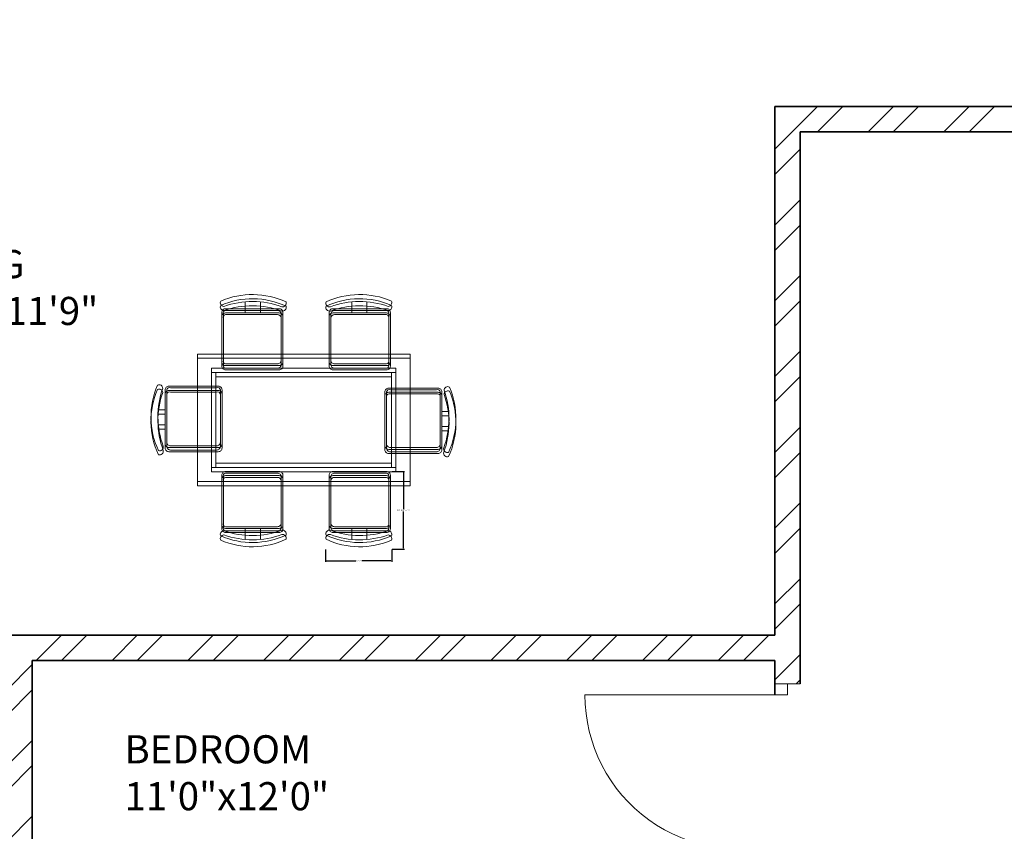
# Model space of a CAD drawing. Units: inches. Extents: x 1885 to 2748, y 783 to 2421.
# Tile 22 of 117: x 2163 to 2338, y 1206 to 1350. Entities that reach past the tile are written whole.
import ezdxf

# ---------------------------------------------------------------- set-up
doc = ezdxf.new("R2010")
doc.units = ezdxf.units.IN
for name, color, linetype, lineweight in [('A-ANNO-DIMS', 2, 'Continuous', 18), ('A-AREA-IDEN', 7, 'Continuous', 18), ('A-DOOR', 31, 'Continuous', 18), ('A-FURN', 8, 'Continuous', 13), ('A-WALL', 7, 'Continuous', 35)]:
    doc.layers.add(name, color=color, linetype=linetype, lineweight=lineweight)
doc.layers.add('A-WALL-PATT', color=85, linetype='Continuous', lineweight=13, true_color=0x58ba48)
doc.styles.get("Standard").update_dxf_attribs({"font": 'arial.ttf'})
doc.dimstyles.get("Standard").update_dxf_attribs({"dimtxt": 0.18, "dimasz": 0.18, "dimexe": 0.18, "dimexo": 0.0625, "dimgap": 0.09, "dimtad": 0, "dimtih": 1, "dimtoh": 1, "dimdec": 4, "dimzin": 0, "dimdsep": 46, "dimtxsty": 'Standard', "dimcen": 0.09, "dimadec": 0, "dimazin": 0, "dimtfac": 1, "dimtdec": 4, "dimtofl": 0, "dimtmove": 0, "dimatfit": 3, "dimfxl": 1, "dimtolj": 1, "dimtzin": 0, "dimarcsym": 0})

# ---------------------------------------------------------------- blocks, each defined once
blk = doc.blocks.new('TABLE-DINING-RECT')
for points in [[(0, 23.42), (37.78, 23.42), (37.78, 0.75), (0, 0.75)], [(0, 23.42), (37.78, 23.42), (37.78, 0.75), (0, 0.75)], [(0, 22.67), (37.78, 22.67), (37.78, 0), (0, 0)], [(0, 22.67), (37.78, 22.67), (37.78, 0), (0, 0)], [(2.51, 20.9), (35.26, 20.9), (35.26, 3.27), (2.51, 3.27)], [(2.51, 20.9), (35.26, 20.9), (35.26, 3.27), (2.51, 3.27)], [(2.51, 20.15), (35.26, 20.15), (35.26, 2.52), (2.51, 2.52)], [(2.51, 20.15), (35.26, 20.15), (35.26, 2.52), (2.51, 2.52)], [(3.27, 20.15), (34.5, 20.15), (34.5, 4.03), (3.27, 4.03)], [(3.27, 20.15), (34.5, 20.15), (34.5, 4.03), (3.27, 4.03)], [(3.27, 19.39), (34.5, 19.39), (34.5, 3.27), (3.27, 3.27)], [(3.27, 19.39), (34.5, 19.39), (34.5, 3.27), (3.27, 3.27)]]:
    blk.add_lwpolyline(points, close=True)
blk = doc.blocks.new('CHAIR-DINING-SIDE')
for points in [[(0.62, 11.29, -0.175809), (10.91, 11.21, 0.578392), (11.69, 12.07, 0.214524), (0.07, 12.23, 0.552014), (0.62, 11.29, -0.065079)], [(0.62, 11.29, -0.175809), (10.91, 11.21, 0.578392), (11.69, 12.07, 0.214524), (0.07, 12.23, 0.552014), (0.62, 11.29, -0.065079)], [(0.62, 10.54, -0.175809), (10.91, 10.46, 0.578392), (11.69, 11.32, 0.214524), (0.07, 11.47, 0.552014), (0.62, 10.54, -0.065079)], [(0.62, 10.54, -0.175809), (10.91, 10.46, 0.578392), (11.69, 11.32, 0.214524), (0.07, 11.47, 0.552014), (0.62, 10.54, -0.065079)], [(10.47, 10.88), (0.92, 10.88, 0.414214), (0.25, 10.21), (0.25, 1.43, 0.414214), (0.92, 0.76), (10.47, 0.76, 0.414214), (11.14, 1.43), (11.14, 10.21, 0.414214), (10.47, 10.88)], [(10.47, 10.88), (0.92, 10.88, 0.414214), (0.25, 10.21), (0.25, 1.43, 0.414214), (0.92, 0.76), (10.47, 0.76, 0.414214), (11.14, 1.43), (11.14, 10.21, 0.414214), (10.47, 10.88)], [(7.12, 10.88), (7.12, 12.09, -0.064759)], [(7.12, 10.88), (7.12, 12.09, -0.064759)], [(7.12, 10.12), (7.12, 11.33, -0.064759)], [(7.12, 10.12), (7.12, 11.33, -0.064759)], [(10.47, 10.12), (0.92, 10.12, 0.414214), (0.25, 9.46), (0.25, 0.67, 0.414214), (0.92, 0), (10.47, 0, 0.414214), (11.14, 0.67), (11.14, 9.46, 0.414214), (10.47, 10.12)], [(10.47, 10.12), (0.92, 10.12, 0.414214), (0.25, 9.46), (0.25, 0.67, 0.414214), (0.92, 0), (10.47, 0, 0.414214), (11.14, 0.67), (11.14, 9.46, 0.414214), (10.47, 10.12)]]:
    blk.add_lwpolyline(points, format="xyb")
for points in [[(0.92, 10.58), (10.17, 10.58, -0.414214), (10.84, 9.91), (10.84, 1.73, -0.414214), (10.17, 1.06), (0.92, 1.06, -0.512069), (0.55, 1.73), (0.55, 9.91, -0.512069)], [(0.92, 10.58), (10.17, 10.58, -0.414214), (10.84, 9.91), (10.84, 1.73, -0.414214), (10.17, 1.06), (0.92, 1.06, -0.512069), (0.55, 1.73), (0.55, 9.91, -0.512069)], [(0.92, 9.82), (10.17, 9.82, -0.414214), (10.84, 9.15), (10.84, 0.97, -0.414214), (10.17, 0.3), (0.92, 0.3, -0.512069), (0.55, 0.97), (0.55, 9.15, -0.512069)], [(0.92, 9.82), (10.17, 9.82, -0.414214), (10.84, 9.15), (10.84, 0.97, -0.414214), (10.17, 0.3), (0.92, 0.3, -0.512069), (0.55, 0.97), (0.55, 9.15, -0.512069)]]:
    blk.add_lwpolyline(points, format="xyb", close=True)
for points in [[(4.44, 12.11), (4.44, 10.88)], [(4.44, 12.11), (4.44, 10.88)], [(4.44, 11.35), (4.44, 10.12)], [(4.44, 11.35), (4.44, 10.12)]]:
    blk.add_lwpolyline(points)
blk = doc.blocks.new('CHAIR-DINING-SIDE-B')
for points in [[(10.8, 3.27, 0.414214), (11.47, 3.94), (11.47, 12.73, 0.414214), (10.8, 13.39), (1.25, 13.39, 0.414214), (0.58, 12.73), (0.58, 3.94, 0.414214), (1.25, 3.27), (10.8, 3.27)], [(10.8, 3.27, 0.414214), (11.47, 3.94), (11.47, 12.73, 0.414214), (10.8, 13.39), (1.25, 13.39, 0.414214), (0.58, 12.73), (0.58, 3.94, 0.414214), (1.25, 3.27), (10.8, 3.27)], [(10.8, 2.52, 0.414214), (11.47, 3.19), (11.47, 11.97, 0.414214), (10.8, 12.64), (1.25, 12.64, 0.414214), (0.58, 11.97), (0.58, 3.19, 0.414214), (1.25, 2.52), (10.8, 2.52)], [(10.8, 2.52, 0.414214), (11.47, 3.19), (11.47, 11.97, 0.414214), (10.8, 12.64), (1.25, 12.64, 0.414214), (0.58, 11.97), (0.58, 3.19, 0.414214), (1.25, 2.52), (10.8, 2.52)], [(11.1, 2.86, -0.175809), (0.81, 2.94, 0.578392), (0.03, 2.08, 0.214524), (11.65, 1.93, 0.552014), (11.1, 2.86, -0.065079)], [(11.1, 2.86, -0.175809), (0.81, 2.94, 0.578392), (0.03, 2.08, 0.214524), (11.65, 1.93, 0.552014), (11.1, 2.86, -0.065079)], [(11.1, 2.11, -0.175809), (0.81, 2.18, 0.578392), (0.03, 1.33, 0.214524), (11.65, 1.17, 0.552014), (11.1, 2.11, -0.065079)], [(11.1, 2.1, -0.175809), (0.81, 2.18, 0.578392), (0.03, 1.33, 0.214524), (11.65, 1.17, 0.552014), (11.1, 2.1, -0.065079)], [(4.6, 3.27), (4.6, 2.07, -0.064759)], [(4.6, 3.27), (4.6, 2.07, -0.064759)], [(4.6, 2.52), (4.6, 1.31, -0.064759)], [(4.6, 2.52), (4.6, 1.31, -0.064759)]]:
    blk.add_lwpolyline(points, format="xyb")
for points in [[(10.8, 3.57), (1.55, 3.57, -0.414214), (0.88, 4.24), (0.88, 12.42, -0.414214), (1.55, 13.09), (10.8, 13.09, -0.512069), (11.17, 12.42), (11.17, 4.24, -0.512069)], [(10.8, 3.57), (1.55, 3.57, -0.414214), (0.88, 4.24), (0.88, 12.42, -0.414214), (1.55, 13.09), (10.8, 13.09, -0.512069), (11.17, 12.42), (11.17, 4.24, -0.512069)], [(10.8, 2.82), (1.55, 2.82, -0.414214), (0.88, 3.49), (0.88, 11.67, -0.414214), (1.55, 12.34), (10.8, 12.34, -0.512069), (11.17, 11.67), (11.17, 3.49, -0.512069)], [(10.8, 2.82), (1.55, 2.82, -0.414214), (0.88, 3.49), (0.88, 11.67, -0.414214), (1.55, 12.34), (10.8, 12.34, -0.512069), (11.17, 11.67), (11.17, 3.49, -0.512069)]]:
    blk.add_lwpolyline(points, format="xyb", close=True)
for points in [[(7.28, 2.04), (7.28, 3.27)], [(7.28, 2.04), (7.28, 3.27)], [(7.28, 1.29), (7.28, 2.52)], [(7.28, 1.29), (7.28, 2.52)]]:
    blk.add_lwpolyline(points)
blk = doc.blocks.new('*D39')
at = {"layer": 'A-ANNO-DIMS', "color": 0, "lineweight": -2, "transparency": 16777216}
for p, q in [((2228.76, 1269.64), (2230.95, 1269.64)), ((2230.77, 1269.46), (2230.77, 1262.91)), ((2230.77, 1255.99), (2230.77, 1262.54)), ((2228.76, 1255.81), (2230.95, 1255.81))]:
    blk.add_line(p, q, dxfattribs=at)
at = {"layer": 'A-ANNO-DIMS', "color": 0, "transparency": 16777216}
for points in [[(2230.74, 1269.46), (2230.8, 1269.46), (2230.77, 1269.64)], [(2230.74, 1255.99), (2230.8, 1255.99), (2230.77, 1255.81)]]:
    blk.add_solid(points, dxfattribs=at)
at = {"layer": 'Defpoints', "color": 0, "transparency": 16777216}
for p in [(2228.7, 1269.64), (2230.77, 1269.64), (2228.7, 1255.81)]:
    blk.add_point(p, dxfattribs=at)
at = {"layer": 'A-ANNO-DIMS', "color": 0, "transparency": 16777216, "insert": (2230.77, 1262.73), "char_height": 0.18, "attachment_point": 5}
blk.add_mtext('\\A1;SIDE CHAIR B 14 TYP.', dxfattribs=at)
blk = doc.blocks.new('*D40')
at = {"layer": 'A-ANNO-DIMS', "color": 0, "lineweight": -2, "transparency": 16777216}
for p, q in [((2216.91, 1255.75), (2216.91, 1253.55)), ((2228.7, 1255.75), (2228.7, 1253.55)), ((2217.09, 1253.73), (2222.28, 1253.73)), ((2228.52, 1253.73), (2223.32, 1253.73))]:
    blk.add_line(p, q, dxfattribs=at)
at = {"layer": 'A-ANNO-DIMS', "color": 0, "transparency": 16777216}
for points in [[(2217.09, 1253.76), (2217.09, 1253.7), (2216.91, 1253.73)], [(2228.52, 1253.76), (2228.52, 1253.7), (2228.7, 1253.73)]]:
    blk.add_solid(points, dxfattribs=at)
at = {"layer": 'Defpoints', "color": 0, "transparency": 16777216}
for p in [(2216.91, 1255.81), (2228.7, 1255.81), (2228.7, 1253.73)]:
    blk.add_point(p, dxfattribs=at)
at = {"layer": 'A-ANNO-DIMS', "color": 0, "transparency": 16777216, "insert": (2222.8, 1253.73), "char_height": 0.18, "attachment_point": 5}
blk.add_mtext('\\A1;12 TYP.', dxfattribs=at)

msp = doc.modelspace()

# ---------------------------------------------------------------- hatches: boundary and pattern name
at = {"layer": 'A-WALL-PATT'}
h = msp.add_hatch(dxfattribs=at)
h.set_pattern_fill('ANSI32', color=256)
h.paths.add_polyline_path([(2007.77, 2318.01), (1980.77, 2318.01), (1980.77, 2281.22), (1985.27, 2281.22), (1985.27, 2313.51), (2007.77, 2313.51), (2007.77, 2315.76)])
h.paths.add_polyline_path([(2094.32, 2318.01), (2067.77, 2318.01), (2067.77, 2313.51), (2094.32, 2313.51), (2094.32, 2315.76)])
h.paths.add_polyline_path([(2131.37, 2315.76), (2131.37, 2318.01), (2131.19, 2318.01), (2112.61, 2318.01), (2112.61, 2313.51), (2117.27, 2313.51), (2117.27, 2255.2), (2121.77, 2255.2), (2121.77, 2313.51), (2131.37, 2313.51)])
h.paths.add_polyline_path([(2190.51, 2318.01), (2155.37, 2318.01), (2155.37, 2313.51), (2169.77, 2313.51), (2169.77, 2229.51), (2121.77, 2229.51), (2121.77, 2233.45), (2119.52, 2233.45), (2117.27, 2233.45), (2117.27, 2201.1), (2121.77, 2201.1), (2121.77, 2225.01), (2169.77, 2225.01), (2169.77, 2165.01), (2306.27, 2165.01), (2306.27, 2066.01), (2310.77, 2066.01), (2344.27, 2066.01), (2486.27, 2066.01), (2486.27, 1886.01), (2483.02, 1886.01), (2483.02, 1881.51), (2486.27, 1881.51), (2486.27, 1880.68), (2490.77, 1880.68), (2490.77, 2070.51), (2344.27, 2070.51), (2310.77, 2070.51), (2310.77, 2165.01), (2310.77, 2173.64), (2308.52, 2173.64), (2306.27, 2173.64), (2306.27, 2169.51), (2174.27, 2169.51), (2174.27, 2313.51), (2190.51, 2313.51), (2190.51, 2315.76)])
h.paths.add_polyline_path([(1985.27, 2221.22), (1980.77, 2221.22), (1980.77, 2165.01), (1992.77, 2165.01), (1992.77, 2141.93), (1997.27, 2141.93), (1997.27, 2165.01), (2117.27, 2165.01), (2117.27, 2163.13), (2121.77, 2163.13), (2121.77, 2172.73), (2119.52, 2172.73), (2117.27, 2172.73), (2117.27, 2169.51), (1985.27, 2169.51)])
h.paths.add_polyline_path([(1997.27, 2105.93), (1992.77, 2105.93), (1992.77, 2070.51), (2016.77, 2070.51), (2016.77, 2059.12), (2019.02, 2059.12), (2021.27, 2059.12), (2021.27, 2070.51), (2117.27, 2070.51), (2117.27, 2022.51), (2114.42, 2022.51), (2114.42, 2018.01), (2123.63, 2018.01), (2123.63, 2020.26), (2123.63, 2022.51), (2121.77, 2022.51), (2121.77, 2142.59), (2119.52, 2142.59), (2117.27, 2142.59), (2117.27, 2075.01), (1997.27, 2075.01)])
h.paths.add_polyline_path([(2092.03, 2020.26), (2092.03, 2022.51), (2021.27, 2022.51), (2021.27, 2035.12), (2016.77, 2035.12), (2016.77, 2018.01), (2016.77, 1978.78), (2021.27, 1978.78), (2021.27, 2018.01), (2092.03, 2018.01)])
h.paths.add_polyline_path([(2260.94, 2022.51), (2153.1, 2022.51), (2153.1, 2020.26), (2153.1, 2018.01), (2155.27, 2018.01), (2155.27, 1886.01), (2107.63, 1886.01), (2107.63, 1881.51), (2182.91, 1881.51), (2182.91, 1883.76), (2182.91, 1886.01), (2159.77, 1886.01), (2159.77, 2018.01), (2260.94, 2018.01), (2260.94, 2020.26)])
h.paths.add_polyline_path([(2047.63, 1883.76), (2047.63, 1886.01), (2021.27, 1886.01), (2021.27, 1918.78), (2019.02, 1918.78), (2016.77, 1918.78), (2016.77, 1881.51), (2047.63, 1881.51)])
h.paths.add_polyline_path([(2306.36, 1883.76), (2306.36, 1886.01), (2296.27, 1886.01), (2296.27, 1982.01), (2316.54, 1982.01), (2316.54, 1984.26), (2316.54, 1986.51), (2296.27, 1986.51), (2296.27, 2022.51), (2289.28, 2022.51), (2289.28, 2018.01), (2291.77, 2018.01), (2291.77, 1886.01), (2242.91, 1886.01), (2242.91, 1881.51), (2306.36, 1881.51)], flags=17)
h.paths.add_polyline_path([(1985.27, 1843.01), (2021.6, 1843.01), (2021.53, 1845.44), (2021.48, 1847.51), (1980.77, 1847.51), (1980.77, 1809.45), (1985.27, 1809.45)])
h.paths.add_polyline_path([(2131.48, 1845.26), (2131.48, 1847.51), (2081.53, 1847.51), (2081.53, 1843.01), (2117.27, 1843.01), (2117.27, 1784.15), (2119.52, 1784.15), (2121.77, 1784.15), (2121.77, 1843.01), (2131.48, 1843.01)])
h.paths.add_polyline_path([(2203.89, 1847.51), (2155.48, 1847.51), (2155.48, 1843.01), (2169.77, 1843.01), (2169.77, 1759.01), (2121.77, 1759.01), (2121.77, 1761.46), (2117.27, 1761.46), (2117.27, 1730.43), (2121.77, 1730.43), (2121.77, 1754.51), (2177.42, 1754.51), (2177.42, 1756.76), (2177.42, 1759.01), (2174.27, 1759.01), (2174.27, 1843.01), (2203.89, 1843.01)])
h.paths.add_polyline_path([(2335.55, 1845.26), (2335.55, 1847.51), (2239.89, 1847.51), (2239.89, 1843.01), (2306.27, 1843.01), (2306.27, 1759.01), (2199.49, 1759.01), (2199.49, 1754.51), (2310.77, 1754.51), (2310.77, 1843.01), (2335.55, 1843.01)])
h.paths.add_polyline_path([(2348.77, 2022.51), (2344.27, 2022.51), (2344.27, 1986.51), (2341.68, 1986.51), (2341.68, 1982.01), (2344.27, 1982.01), (2344.27, 1886.01), (2330.36, 1886.01), (2330.36, 1881.51), (2361.63, 1881.51), (2361.63, 1883.76), (2361.63, 1886.01), (2348.77, 1886.01)], flags=17)
h.paths.add_polyline_path([(2283.25, 2315.76), (2283.25, 2318.01), (2238.51, 2318.01), (2238.51, 2313.51), (2283.25, 2313.51)], flags=17)
h.paths.add_polyline_path([(2363.27, 2348.01), (2388.68, 2348.01), (2388.68, 2350.26), (2388.68, 2352.51), (2358.77, 2352.51), (2358.77, 2348.01), (2358.77, 2318.01), (2344.48, 2318.01), (2344.48, 2313.51), (2358.77, 2313.51), (2358.77, 2229.51), (2310.77, 2229.51), (2310.77, 2231.95), (2306.27, 2231.95), (2306.27, 2205.61), (2310.77, 2205.61), (2310.77, 2225.01), (2358.77, 2225.01), (2358.77, 2211.51), (2452.33, 2211.51), (2452.33, 2213.76), (2452.33, 2216.01), (2363.27, 2216.01), (2363.27, 2318.01)])
h.paths.add_polyline_path([(2310.77, 2313.51), (2320.48, 2313.51), (2320.48, 2315.76), (2320.48, 2318.01), (2302.73, 2318.01), (2302.73, 2313.51), (2306.27, 2313.51), (2306.27, 2251.08), (2310.77, 2251.08)], flags=17)
h.paths.add_polyline_path([(2490.77, 2352.51), (2486.27, 2352.51), (2448.68, 2352.51), (2448.68, 2348.01), (2486.27, 2348.01), (2486.27, 2318.01), (2486.27, 2216.01), (2481.78, 2216.01), (2481.78, 2211.51), (2486.27, 2211.51), (2486.27, 2165.01), (2493.29, 2165.01), (2493.29, 2167.26), (2493.29, 2169.51), (2490.77, 2169.51), (2490.77, 2313.51), (2494.43, 2313.51), (2494.43, 2318.01), (2490.77, 2318.01)])
h.paths.add_polyline_path([(2534.65, 2318.01), (2515.69, 2318.01), (2515.69, 2313.51), (2534.65, 2313.51), (2534.65, 2315.76)])
h.paths.add_polyline_path([(2618.27, 2318.01), (2594.65, 2318.01), (2594.65, 2313.51), (2613.77, 2313.51), (2613.77, 2281.71), (2618.27, 2281.71)])
h.paths.add_polyline_path([(2618.27, 2221.71), (2613.77, 2221.71), (2613.77, 2169.51), (2554.02, 2169.51), (2554.02, 2165.01), (2613.77, 2165.01), (2613.77, 2152.88), (2618.27, 2152.88)])
h.paths.add_polyline_path([(2618.27, 2128.88), (2616.02, 2128.88), (2613.77, 2128.88), (2613.77, 2117.01), (2529.77, 2117.01), (2529.77, 2165.01), (2532.85, 2165.01), (2532.85, 2169.51), (2522.87, 2169.51), (2522.87, 2165.01), (2525.27, 2165.01), (2525.27, 2117.01), (2525.27, 2112.51), (2525.27, 2108.58), (2529.77, 2108.58), (2529.77, 2112.51), (2613.77, 2112.51), (2613.77, 2080.19), (2618.27, 2080.19)])
h.paths.add_polyline_path([(2618.27, 2044.19), (2616.02, 2044.19), (2613.77, 2044.19), (2613.77, 2015.51), (2529.77, 2015.51), (2529.77, 2088.58), (2527.52, 2088.58), (2525.27, 2088.58), (2525.27, 2011.01), (2613.77, 2011.01), (2613.77, 1956.75), (2618.27, 1956.75)])
h.paths.add_polyline_path([(2618.27, 1881.51), (2618.27, 1896.75), (2613.77, 1896.75), (2613.77, 1881.51), (2613.77, 1847.51), (2592.71, 1847.51), (2592.71, 1843.01), (2613.77, 1843.01), (2613.77, 1765.01), (2613.77, 1760.51), (2609.62, 1760.51), (2609.62, 1756.01), (2613.77, 1756.01), (2613.77, 1660.01), (2608.54, 1660.01), (2608.54, 1655.51), (2613.77, 1655.51), (2613.77, 1508.16), (2618.27, 1508.16)])
h.paths.add_polyline_path([(2565.77, 1843.01), (2569, 1843.01), (2569, 1847.51), (2490.77, 1847.51), (2490.77, 1849.7), (2488.52, 1849.7), (2486.27, 1849.7), (2486.27, 1847.51), (2477.27, 1847.51), (2477.27, 1838.51), (2477.27, 1821.49), (2486.27, 1821.49), (2486.27, 1838.51), (2561.27, 1838.51), (2561.27, 1765.01), (2486.27, 1765.01), (2486.27, 1786.16), (2477.27, 1786.16), (2477.27, 1765.01), (2477.27, 1756.01), (2486.27, 1756.01), (2565.77, 1756.01), (2585.62, 1756.01), (2585.62, 1758.26), (2585.62, 1760.51), (2565.77, 1760.51), (2565.77, 1765.01)])
h.paths.add_polyline_path([(2486.27, 1651.01), (2561.27, 1651.01), (2561.27, 1567.01), (2486.27, 1567.01), (2486.27, 1591.32), (2477.27, 1591.32), (2477.27, 1567.01), (2477.27, 1558.01), (2477.27, 1555.44), (2481.77, 1555.44), (2481.77, 1558.01), (2568.65, 1558.01), (2568.65, 1560.26), (2568.65, 1562.51), (2565.77, 1562.51), (2565.77, 1655.51), (2584.54, 1655.51), (2584.54, 1657.76), (2584.54, 1660.01), (2565.77, 1660.01), (2486.27, 1660.01), (2477.27, 1660.01), (2477.27, 1651.01), (2477.27, 1632.99), (2486.27, 1632.99)])
h.paths.add_polyline_path([(2449.97, 1883.76), (2449.97, 1886.01), (2421.63, 1886.01), (2421.63, 1881.51), (2449.97, 1881.51)], flags=17)
h.paths.add_polyline_path([(2447.27, 1847.51), (2395.55, 1847.51), (2395.55, 1843.01), (2442.77, 1843.01), (2442.77, 1809.27), (2447.27, 1809.27)])
h.paths.add_polyline_path([(1985.27, 1749.45), (1980.77, 1749.45), (1980.77, 1694.5), (1985.27, 1694.5), (1985.27, 1694.51), (1986.9, 1694.51), (1986.9, 1697.78), (1986.9, 1699.01), (1985.27, 1699.01)])
h.paths.add_polyline_path([(2152.77, 1699.01), (2121.77, 1699.01), (2121.77, 1703.67), (2119.52, 1703.67), (2117.27, 1703.67), (2117.27, 1699.01), (2009.22, 1699.01), (2009.22, 1694.51), (2148.27, 1694.51), (2148.27, 1692.63), (2152.77, 1692.63)])
h.paths.add_polyline_path([(2016.27, 1694.51), (2011.77, 1694.51), (2011.77, 1558.01), (2040.81, 1558.01), (2040.81, 1560.26), (2040.81, 1562.51), (2016.27, 1562.51)])
h.paths.add_polyline_path([(2152.77, 1663.02), (2150.52, 1663.02), (2148.27, 1663.02), (2148.27, 1562.51), (2100.81, 1562.51), (2100.81, 1558.01), (2165.12, 1558.01), (2165.12, 1560.26), (2165.12, 1562.51), (2152.77, 1562.51), (2152.77, 1610.51), (2224.77, 1610.51), (2224.77, 1607.99), (2229.27, 1607.99), (2229.27, 1615.01), (2152.77, 1615.01)])
h.paths.add_polyline_path([(2238.61, 1560.26), (2238.61, 1562.51), (2229.27, 1562.51), (2229.27, 1588.76), (2227.02, 1588.76), (2224.77, 1588.77), (2224.77, 1562.51), (2189.12, 1562.51), (2189.12, 1558.01), (2238.61, 1558.01)])
h.paths.add_polyline_path([(2336.02, 1560.26), (2336.02, 1562.51), (2310.77, 1562.51), (2310.77, 1656.35), (2308.52, 1656.35), (2306.27, 1656.35), (2306.27, 1562.51), (2286.61, 1562.51), (2286.61, 1558.01), (2336.02, 1558.01)])
h.paths.add_polyline_path([(2447.27, 1690.97), (2445.02, 1690.97), (2442.77, 1690.97), (2442.77, 1687.01), (2306.27, 1687.01), (2306.27, 1680.75), (2310.77, 1680.75), (2310.77, 1682.51), (2442.77, 1682.51), (2442.77, 1562.51), (2396.02, 1562.51), (2396.02, 1558.01), (2447.27, 1558.01)])
h.paths.add_polyline_path([(2447.27, 1749.27), (2445.02, 1749.27), (2442.77, 1749.27), (2442.77, 1717.23), (2447.27, 1717.23)])
h.paths.add_polyline_path([(2044.67, 1521.76), (2044.67, 1524.01), (2007.27, 1524.01), (2007.27, 1503.49), (2009.52, 1503.49), (2011.77, 1503.49), (2011.77, 1519.51), (2044.67, 1519.51)])
h.paths.add_polyline_path([(2177.97, 1521.76), (2177.97, 1524.01), (2104.67, 1524.01), (2104.67, 1519.51), (2145.77, 1519.51), (2145.77, 1387.51), (2143.37, 1387.51), (2143.37, 1383.01), (2251.59, 1383.01), (2251.59, 1385.26), (2251.59, 1387.51), (2150.27, 1387.51), (2150.27, 1519.51), (2177.97, 1519.51)])
h.paths.add_polyline_path([(2298.7, 1524.01), (2237.97, 1524.01), (2237.97, 1519.51), (2282.27, 1519.51), (2282.27, 1387.51), (2279.68, 1387.51), (2279.68, 1383.01), (2286.77, 1383.01), (2286.77, 1419.01), (2312.45, 1419.01), (2312.45, 1421.26), (2312.45, 1423.51), (2286.77, 1423.51), (2286.77, 1519.51), (2298.7, 1519.51), (2298.7, 1521.72)], flags=17)
h.paths.add_polyline_path([(2361.9, 1521.76), (2361.9, 1524.01), (2322.7, 1524.01), (2322.7, 1519.51), (2334.77, 1519.51), (2334.77, 1423.51), (2331.93, 1423.51), (2331.93, 1419.01), (2334.77, 1419.01), (2334.77, 1387.51), (2334.77, 1383.23), (2339.27, 1383.23), (2339.27, 1387.51), (2339.27, 1519.51), (2361.9, 1519.51)], flags=17)
h.paths.add_polyline_path([(2447.27, 1521.76), (2447.27, 1524.01), (2421.9, 1524.01), (2421.9, 1519.51), (2447.27, 1519.51)], flags=17)
h.paths.add_polyline_path([(2481.77, 1529.6), (2479.52, 1529.6), (2477.27, 1529.6), (2477.27, 1524.01), (2474.49, 1524.01), (2474.49, 1519.51), (2477.27, 1519.51), (2477.27, 1334.51), (2296.77, 1334.51), (2296.77, 1240.51), (2160.27, 1240.51), (2160.27, 1180.51), (2112.27, 1180.51), (2112.27, 1207.69), (2110.02, 1207.69), (2107.77, 1207.69), (2107.77, 1171.61), (2112.27, 1171.61), (2112.27, 1176.01), (2160.27, 1176.01), (2160.27, 1092.01), (2144.22, 1092.01), (2144.22, 1087.51), (2189.5, 1087.51), (2189.5, 1089.76), (2189.5, 1092.01), (2164.77, 1092.01), (2164.77, 1236.01), (2296.77, 1236.01), (2296.77, 1231.91), (2301.27, 1231.91), (2301.27, 1330.01), (2481.77, 1330.01), (2481.77, 1387.51)])
h.paths.add_polyline_path([(2618.27, 1448.16), (2613.77, 1448.16), (2613.77, 1382.51), (2529.77, 1382.51), (2525.27, 1382.51), (2525.27, 1307.06), (2529.77, 1307.06), (2529.77, 1378.01), (2613.77, 1378.01), (2613.77, 1354.99), (2618.27, 1354.99)])
h.paths.add_polyline_path([(2618.27, 1318.99), (2613.77, 1318.99), (2613.77, 1281.01), (2529.77, 1281.01), (2529.77, 1283.79), (2527.52, 1283.79), (2525.27, 1283.79), (2525.27, 1228.51), (2516.79, 1228.51), (2516.79, 1224.01), (2533.48, 1224.01), (2533.48, 1226.26), (2533.48, 1228.51), (2529.77, 1228.51), (2529.77, 1276.51), (2613.77, 1276.51), (2613.77, 1266.02), (2618.27, 1266.02)])
h.paths.add_polyline_path([(2618.27, 1134.96), (2613.77, 1134.96), (2613.77, 1092.01), (2594.54, 1092.01), (2594.54, 1087.51), (2618.27, 1087.51)])
h.paths.add_polyline_path([(2534.54, 1092.01), (2509.77, 1092.01), (2509.77, 1087.51), (2534.54, 1087.51), (2534.54, 1089.76)])
h.paths.add_polyline_path([(2481.27, 1224.01), (2484.12, 1224.01), (2484.12, 1226.26), (2484.12, 1228.51), (2476.77, 1228.51), (2476.77, 1198.51), (2471.61, 1198.51), (2471.61, 1194.01), (2476.77, 1194.01), (2476.77, 1062.01), (2436.89, 1062.01), (2436.89, 1057.51), (2476.77, 1057.51), (2481.27, 1057.51), (2481.27, 1062.01), (2481.27, 1087.51), (2485.35, 1087.51), (2485.35, 1089.76), (2485.35, 1092.01), (2481.27, 1092.01), (2481.27, 1117.51)])
h.paths.add_polyline_path([(2439.9, 1198.51), (2349.27, 1198.51), (2349.27, 1194.01), (2349.27, 1180.51), (2301.27, 1180.51), (2301.27, 1201.9), (2299.02, 1201.9), (2296.77, 1201.9), (2296.77, 1172.34), (2299.02, 1172.34), (2301.27, 1172.34), (2301.27, 1176.01), (2349.27, 1176.01), (2349.27, 1092.01), (2334.45, 1092.01), (2334.45, 1087.51), (2349.27, 1087.51), (2349.27, 1057.51), (2353.77, 1057.51), (2376.89, 1057.51), (2376.89, 1059.76), (2376.89, 1062.01), (2353.77, 1062.01), (2353.77, 1087.51), (2353.77, 1180.51), (2353.77, 1194.01), (2439.9, 1194.01), (2439.9, 1196.26)])
h.paths.add_polyline_path([(2270.6, 1089.76), (2270.6, 1092.01), (2249.5, 1092.01), (2249.5, 1087.51), (2270.6, 1087.51)], flags=17)
h.paths.add_polyline_path([(2310.45, 1092.01), (2301.27, 1092.01), (2301.27, 1153.29), (2296.77, 1153.29), (2296.77, 1092.01), (2293.79, 1092.01), (2293.79, 1087.51), (2310.45, 1087.51), (2310.45, 1089.76)], flags=17)
h.paths.add_polyline_path([(2112.27, 1150.33), (2110.02, 1150.33), (2107.77, 1150.33), (2107.77, 1092.01), (2104.47, 1092.01), (2104.47, 1087.51), (2120.22, 1087.51), (2120.22, 1089.76), (2120.22, 1092.01), (2112.27, 1092.01)])
h.paths.add_polyline_path([(2082.17, 1092.01), (2058.14, 1092.01), (2058.14, 1087.51), (2082.17, 1087.51), (2082.17, 1089.76)])
h.paths.add_polyline_path([(1975.77, 1145.64), (1971.27, 1145.64), (1971.27, 1087.51), (1980.77, 1087.51), (1998.14, 1087.51), (1998.14, 1089.76), (1998.14, 1092.01), (1985.27, 1092.01), (1975.77, 1092.01)])
h.paths.add_polyline_path([(2112.27, 1244.38), (2110.02, 1244.38), (2107.77, 1244.38), (2107.77, 1240.51), (1992.27, 1240.51), (1992.27, 1271.01), (1987.77, 1271.01), (1987.77, 1240.51), (1980.77, 1240.51), (1975.77, 1240.51), (1971.27, 1240.51), (1971.27, 1205.64), (1975.77, 1205.64), (1975.77, 1236.01), (2107.77, 1236.01), (2107.77, 1233.44), (2112.27, 1233.44), (2112.27, 1236.01)])
h.paths.add_polyline_path([(2112.27, 1383.01), (2114.78, 1383.01), (2114.78, 1385.26), (2114.78, 1387.51), (2102.48, 1387.51), (2102.48, 1383.01), (2107.77, 1383.01), (2107.77, 1335.01), (2011.77, 1335.01), (2011.77, 1349.94), (2007.27, 1349.94), (2007.27, 1335.01), (1987.77, 1335.01), (1987.77, 1330.51), (1987.77, 1307.01), (1992.27, 1307.01), (1992.27, 1330.51), (2007.27, 1330.51), (2107.77, 1330.51), (2107.77, 1264.71), (2112.27, 1264.71)])
h.paths.add_polyline_path([(2077.86, 1387.51), (2011.77, 1387.51), (2011.77, 1390.04), (2009.52, 1390.04), (2007.27, 1390.04), (2007.27, 1373.94), (2011.77, 1373.94), (2011.77, 1383.01), (2077.86, 1383.01)])
h.paths.add_polyline_path([(2011.77, 1443.49), (2007.27, 1443.49), (2007.27, 1410.25), (2011.77, 1410.25)])

# ---------------------------------------------------------------- linework, layer by layer
at = {"layer": 'A-DOOR'}
for p, q in [((2296.77, 1231.91), (2301.27, 1231.91)), ((2301.27, 1231.91), (2299.02, 1231.91)), ((2299.02, 1231.91), (2299.02, 1229.91)), ((2299.02, 1229.91), (2263.02, 1229.91))]:
    msp.add_line(p, q, dxfattribs=at)
msp.add_arc((2290.42, 1229.91), 27.4, 180, 288.2911, dxfattribs=at)
at = {"layer": 'A-FURN'}
for points in [[(2217.76, 1298.9, -0.578392), (2216.98, 1299.76, -0.214524), (2228.6, 1299.92, -0.552014), (2228.05, 1298.98, 0.175809), (2217.76, 1298.9)], [(2217.76, 1298.9, -0.578392), (2216.98, 1299.76, -0.214524), (2228.6, 1299.92, -0.552014), (2228.05, 1298.98, 0.175809), (2217.76, 1298.9)], [(2217.76, 1298.15, -0.578392), (2216.98, 1299.01, -0.214524), (2228.6, 1299.16, -0.552014), (2228.05, 1298.23, 0.175809), (2217.76, 1298.15)], [(2217.76, 1298.15, -0.578392), (2216.98, 1299.01, -0.214524), (2228.6, 1299.16, -0.552014), (2228.05, 1298.23, 0.175809), (2217.76, 1298.15)], [(2221.55, 1298.57), (2221.55, 1299.78, 0.064759)], [(2221.55, 1298.57), (2221.55, 1299.78, 0.064759)], [(2221.55, 1297.81), (2221.55, 1299.02, 0.064759)], [(2221.55, 1297.81), (2221.55, 1299.02, 0.064759)], [(2227.75, 1298.57, -0.414214), (2228.42, 1297.9), (2228.42, 1289.12, -0.414214), (2227.75, 1288.45), (2218.2, 1288.45, -0.414214), (2217.53, 1289.12), (2217.53, 1297.9, -0.414214), (2218.2, 1298.57), (2227.75, 1298.57)], [(2227.75, 1298.57, -0.414214), (2228.42, 1297.9), (2228.42, 1289.12, -0.414214), (2227.75, 1288.45), (2218.2, 1288.45, -0.414214), (2217.53, 1289.12), (2217.53, 1297.9, -0.414214), (2218.2, 1298.57), (2227.75, 1298.57)], [(2227.75, 1297.81, -0.414214), (2228.42, 1297.15), (2228.42, 1288.36, -0.414214), (2227.75, 1287.69), (2218.2, 1287.69, -0.414214), (2217.53, 1288.36), (2217.53, 1297.15, -0.414214), (2218.2, 1297.81), (2227.75, 1297.81)], [(2227.75, 1297.81, -0.414214), (2228.42, 1297.15), (2228.42, 1288.36, -0.414214), (2227.75, 1287.69), (2218.2, 1287.69, -0.414214), (2217.53, 1288.36), (2217.53, 1297.15, -0.414214), (2218.2, 1297.81), (2227.75, 1297.81)], [(2188.04, 1274.13, -0.578392), (2187.18, 1273.35, -0.214524), (2187.03, 1284.97, -0.552014), (2187.96, 1284.42, 0.175809), (2188.04, 1274.13)], [(2188.04, 1274.13, -0.578392), (2187.18, 1273.35, -0.214524), (2187.03, 1284.97, -0.552014), (2187.96, 1284.42, 0.175809), (2188.04, 1274.13)], [(2188.04, 1273.38, -0.578392), (2187.18, 1272.6, -0.214524), (2187.03, 1284.21, -0.552014), (2187.96, 1283.67, 0.175809), (2188.04, 1273.38)], [(2188.04, 1273.38, -0.578392), (2187.18, 1272.6, -0.214524), (2187.03, 1284.21, -0.552014), (2187.96, 1283.67, 0.175809), (2188.04, 1273.38)], [(2188.38, 1284.12, -0.414214), (2189.05, 1284.79), (2197.83, 1284.79, -0.414214), (2198.5, 1284.12), (2198.5, 1274.57, -0.414214), (2197.83, 1273.9), (2189.05, 1273.9, -0.414214), (2188.38, 1274.57), (2188.38, 1284.12)], [(2188.38, 1284.12, -0.414214), (2189.05, 1284.79), (2197.83, 1284.79, -0.414214), (2198.5, 1284.12), (2198.5, 1274.57, -0.414214), (2197.83, 1273.9), (2189.05, 1273.9, -0.414214), (2188.38, 1274.57), (2188.38, 1284.12)], [(2188.38, 1283.37, -0.414214), (2189.05, 1284.04), (2197.83, 1284.04, -0.414214), (2198.5, 1283.37), (2198.5, 1273.81, -0.414214), (2197.83, 1273.15), (2189.05, 1273.15, -0.414214), (2188.38, 1273.81), (2188.38, 1283.37)], [(2188.38, 1283.37, -0.414214), (2189.05, 1284.04), (2197.83, 1284.04, -0.414214), (2198.5, 1283.37), (2198.5, 1273.81, -0.414214), (2197.83, 1273.15), (2189.05, 1273.15, -0.414214), (2188.38, 1273.81), (2188.38, 1283.37)], [(2237.57, 1283.8, 0.414214), (2236.9, 1284.46), (2228.12, 1284.46, 0.414214), (2227.45, 1283.8), (2227.45, 1274.24, 0.414214), (2228.12, 1273.57), (2236.9, 1273.57, 0.414214), (2237.57, 1274.24), (2237.57, 1283.8)], [(2237.57, 1283.8, 0.414214), (2236.9, 1284.46), (2228.12, 1284.46, 0.414214), (2227.45, 1283.8), (2227.45, 1274.24, 0.414214), (2228.12, 1273.57), (2236.9, 1273.57, 0.414214), (2237.57, 1274.24), (2237.57, 1283.8)], [(2237.57, 1283.04, 0.414214), (2236.9, 1283.71), (2228.12, 1283.71, 0.414214), (2227.45, 1283.04), (2227.45, 1273.49, 0.414214), (2228.12, 1272.82), (2236.9, 1272.82, 0.414214), (2237.57, 1273.49), (2237.57, 1283.04)], [(2237.57, 1283.04, 0.414214), (2236.9, 1283.71), (2228.12, 1283.71, 0.414214), (2227.45, 1283.04), (2227.45, 1273.49, 0.414214), (2228.12, 1272.82), (2236.9, 1272.82, 0.414214), (2237.57, 1273.49), (2237.57, 1283.04)], [(2237.98, 1284.1, -0.175809), (2237.91, 1273.81, 0.578392), (2238.76, 1273.03, 0.214524), (2238.92, 1284.64, 0.552014), (2237.98, 1284.1, -0.065079)], [(2237.98, 1284.1, -0.175809), (2237.91, 1273.81, 0.578392), (2238.76, 1273.03, 0.214524), (2238.92, 1284.64, 0.552014), (2237.98, 1284.1, -0.065079)], [(2237.98, 1283.34, -0.175809), (2237.91, 1273.05, 0.578392), (2238.76, 1272.27, 0.214524), (2238.92, 1283.89, 0.552014), (2237.98, 1283.34, -0.065079)], [(2237.98, 1283.34, -0.175809), (2237.91, 1273.05, 0.578392), (2238.76, 1272.27, 0.214524), (2238.92, 1283.89, 0.552014), (2237.98, 1283.34, -0.065079)], [(2188.38, 1277.93), (2187.17, 1277.93, 0.064759)], [(2188.38, 1277.93), (2187.17, 1277.93, 0.064759)], [(2188.38, 1277.17), (2187.17, 1277.17, 0.064759)], [(2188.38, 1277.17), (2187.17, 1277.17, 0.064759)], [(2237.57, 1277.6), (2238.78, 1277.6, -0.064759)], [(2237.57, 1277.6), (2238.78, 1277.6, -0.064759)], [(2237.57, 1276.84), (2238.78, 1276.84, -0.064759)], [(2237.57, 1276.84), (2238.78, 1276.84, -0.064759)], [(2208.66, 1259.52), (2199.11, 1259.52, -0.414214), (2198.44, 1260.19), (2198.44, 1268.98, -0.414214), (2199.11, 1269.64), (2208.66, 1269.64, -0.414214), (2209.33, 1268.98), (2209.33, 1260.19, -0.414214), (2208.66, 1259.52)], [(2208.66, 1259.52), (2199.11, 1259.52, -0.414214), (2198.44, 1260.19), (2198.44, 1268.98, -0.414214), (2199.11, 1269.64), (2208.66, 1269.64, -0.414214), (2209.33, 1268.98), (2209.33, 1260.19, -0.414214), (2208.66, 1259.52)], [(2208.66, 1258.77), (2199.11, 1258.77, -0.414214), (2198.44, 1259.44), (2198.44, 1268.22, -0.414214), (2199.11, 1268.89), (2208.66, 1268.89, -0.414214), (2209.33, 1268.22), (2209.33, 1259.44, -0.414214), (2208.66, 1258.77)], [(2208.66, 1258.77), (2199.11, 1258.77, -0.414214), (2198.44, 1259.44), (2198.44, 1268.22, -0.414214), (2199.11, 1268.89), (2208.66, 1268.89, -0.414214), (2209.33, 1268.22), (2209.33, 1259.44, -0.414214), (2208.66, 1258.77)], [(2209.1, 1259.19, -0.578392), (2209.88, 1258.33, -0.214524), (2198.26, 1258.18, -0.552014), (2198.81, 1259.11, 0.175809), (2209.1, 1259.19)], [(2209.1, 1259.19, -0.578392), (2209.88, 1258.33, -0.214524), (2198.26, 1258.18, -0.552014), (2198.81, 1259.11, 0.175809), (2209.1, 1259.19)], [(2205.31, 1259.52), (2205.31, 1258.32, 0.064759)], [(2205.31, 1259.52), (2205.31, 1258.32, 0.064759)], [(2205.31, 1258.77), (2205.31, 1257.56, 0.064759)], [(2205.31, 1258.77), (2205.31, 1257.56, 0.064759)], [(2209.1, 1258.43, -0.578392), (2209.88, 1257.58, -0.214524), (2198.26, 1257.42, -0.552014), (2198.81, 1258.36, 0.175809), (2209.1, 1258.43)], [(2209.1, 1258.43, -0.578392), (2209.88, 1257.58, -0.214524), (2198.26, 1257.42, -0.552014), (2198.81, 1258.35, 0.175809), (2209.1, 1258.43)]]:
    msp.add_lwpolyline(points, format="xyb", dxfattribs=at)
for points in [[(2224.23, 1299.8), (2224.23, 1298.57)], [(2224.23, 1299.8), (2224.23, 1298.57)], [(2224.23, 1299.04), (2224.23, 1297.81)], [(2224.23, 1299.04), (2224.23, 1297.81)], [(2187.15, 1280.6), (2188.38, 1280.6)], [(2187.15, 1280.6), (2188.38, 1280.6)], [(2187.15, 1279.84), (2188.38, 1279.84)], [(2187.15, 1279.84), (2188.38, 1279.84)], [(2238.8, 1280.27), (2237.57, 1280.27)], [(2238.8, 1280.27), (2237.57, 1280.27)], [(2238.8, 1279.52), (2237.57, 1279.52)], [(2238.8, 1279.52), (2237.57, 1279.52)], [(2202.63, 1258.29), (2202.63, 1259.52)], [(2202.63, 1258.29), (2202.63, 1259.52)], [(2202.63, 1257.54), (2202.63, 1258.77)], [(2202.63, 1257.54), (2202.63, 1258.77)]]:
    msp.add_lwpolyline(points, dxfattribs=at)
for points in [[(2227.75, 1298.27), (2218.5, 1298.27, 0.414214), (2217.83, 1297.6), (2217.83, 1289.42, 0.414214), (2218.5, 1288.75), (2227.75, 1288.75, 0.512069), (2228.12, 1289.42), (2228.12, 1297.6, 0.512069)], [(2227.75, 1298.27), (2218.5, 1298.27, 0.414214), (2217.83, 1297.6), (2217.83, 1289.42, 0.414214), (2218.5, 1288.75), (2227.75, 1288.75, 0.512069), (2228.12, 1289.42), (2228.12, 1297.6, 0.512069)], [(2227.75, 1297.51), (2218.5, 1297.51, 0.414214), (2217.83, 1296.84), (2217.83, 1288.66, 0.414214), (2218.5, 1287.99), (2227.75, 1287.99, 0.512069), (2228.12, 1288.66), (2228.12, 1296.84, 0.512069)], [(2227.75, 1297.51), (2218.5, 1297.51, 0.414214), (2217.83, 1296.84), (2217.83, 1288.66, 0.414214), (2218.5, 1287.99), (2227.75, 1287.99, 0.512069), (2228.12, 1288.66), (2228.12, 1296.84, 0.512069)], [(2188.68, 1284.12), (2188.68, 1274.87, 0.414214), (2189.35, 1274.2), (2197.53, 1274.2, 0.414214), (2198.2, 1274.87), (2198.2, 1284.12, 0.512069), (2197.53, 1284.49), (2189.35, 1284.49, 0.512069)], [(2188.68, 1284.12), (2188.68, 1274.87, 0.414214), (2189.35, 1274.2), (2197.53, 1274.2, 0.414214), (2198.2, 1274.87), (2198.2, 1284.12, 0.512069), (2197.53, 1284.49), (2189.35, 1284.49, 0.512069)], [(2188.68, 1283.36), (2188.68, 1274.12, 0.414214), (2189.35, 1273.45), (2197.53, 1273.45, 0.414214), (2198.2, 1274.12), (2198.2, 1283.36, 0.512069), (2197.53, 1283.73), (2189.35, 1283.73, 0.512069)], [(2188.68, 1283.36), (2188.68, 1274.12, 0.414214), (2189.35, 1273.45), (2197.53, 1273.45, 0.414214), (2198.2, 1274.12), (2198.2, 1283.36, 0.512069), (2197.53, 1283.73), (2189.35, 1283.73, 0.512069)], [(2237.27, 1283.79), (2237.27, 1274.54, -0.414214), (2236.6, 1273.88), (2228.42, 1273.88, -0.414214), (2227.75, 1274.54), (2227.75, 1283.79, -0.512069), (2228.42, 1284.16), (2236.6, 1284.16, -0.512069)], [(2237.27, 1283.79), (2237.27, 1274.54, -0.414214), (2236.6, 1273.88), (2228.42, 1273.88, -0.414214), (2227.75, 1274.54), (2227.75, 1283.79, -0.512069), (2228.42, 1284.16), (2236.6, 1284.16, -0.512069)], [(2237.27, 1283.04), (2237.27, 1273.79, -0.414214), (2236.6, 1273.12), (2228.42, 1273.12, -0.414214), (2227.75, 1273.79), (2227.75, 1283.04, -0.512069), (2228.42, 1283.41), (2236.6, 1283.41, -0.512069)], [(2237.27, 1283.04), (2237.27, 1273.79, -0.414214), (2236.6, 1273.12), (2228.42, 1273.12, -0.414214), (2227.75, 1273.79), (2227.75, 1283.04, -0.512069), (2228.42, 1283.41), (2236.6, 1283.41, -0.512069)], [(2199.11, 1259.82), (2208.36, 1259.82, 0.414214), (2209.03, 1260.49), (2209.03, 1268.67, 0.414214), (2208.36, 1269.34), (2199.11, 1269.34, 0.512069), (2198.74, 1268.67), (2198.74, 1260.49, 0.512069)], [(2199.11, 1259.82), (2208.36, 1259.82, 0.414214), (2209.03, 1260.49), (2209.03, 1268.67, 0.414214), (2208.36, 1269.34), (2199.11, 1269.34, 0.512069), (2198.74, 1268.67), (2198.74, 1260.49, 0.512069)], [(2199.11, 1259.07), (2208.36, 1259.07, 0.414214), (2209.03, 1259.74), (2209.03, 1267.92, 0.414214), (2208.36, 1268.59), (2199.11, 1268.59, 0.512069), (2198.74, 1267.92), (2198.74, 1259.74, 0.512069)], [(2199.11, 1259.07), (2208.36, 1259.07, 0.414214), (2209.03, 1259.74), (2209.03, 1267.92, 0.414214), (2208.36, 1268.59), (2199.11, 1268.59, 0.512069), (2198.74, 1267.92), (2198.74, 1259.74, 0.512069)]]:
    msp.add_lwpolyline(points, format="xyb", close=True, dxfattribs=at)
at = {"layer": 'A-WALL'}
for p, q in [((2296.77, 1334.51), (2296.77, 1240.51)), ((2477.27, 1334.51), (2296.77, 1334.51)), ((2334.77, 1334.51), (2296.77, 1334.51)), ((2301.27, 1330.01), (2301.27, 1231.91)), ((2301.27, 1330.01), (2481.77, 1330.01)), ((2296.77, 1240.51), (2160.27, 1240.51)), ((2296.77, 1236.01), (2164.77, 1236.01)), ((2164.77, 1236.01), (2164.77, 1092.01)), ((2296.77, 1236.01), (2296.77, 1229.91))]:
    msp.add_line(p, q, dxfattribs=at)

# ---------------------------------------------------------------- block references
at = {"layer": 'A-FURN'}
for name, p in [('CHAIR-DINING-SIDE', (2198.19, 1287.69)), ('TABLE-DINING-RECT', (2194.14, 1267.08)), ('CHAIR-DINING-SIDE-B', (2216.95, 1256.25))]:
    msp.add_blockref(name, p, dxfattribs=at)

# ---------------------------------------------------------------- texts
at = {"layer": 'A-AREA-IDEN', "char_height": 5, "attachment_point": 1}
for s, width, insert in [('DINING\\P15\'7"x11\'9"', 116.7406, (2140.13, 1309)), ('BEDROOM\\P11\'0"x12\'0"', 183.7908, (2181.16, 1222.75))]:
    msp.add_mtext_dynamic_manual_height_columns(s, width=width, gutter_width=12.5, heights=[0], dxfattribs=dict(at, insert=insert))

# ---------------------------------------------------------------- dimensions: what is measured, and where the dimension line sits
at = {"layer": 'A-ANNO-DIMS'}
dim = msp.add_linear_dim(base=(2230.77, 1269.64), p1=(2228.7, 1255.81), p2=(2228.7, 1269.64), angle=90, text='SIDE CHAIR B <> TYP.', dimstyle='Standard', override={"dimdec": 0, "dimlfac": 1, "dimrnd": 0, "dimzin": 0, "dimdsep": 46, "dimlunit": 2}, dxfattribs=at)
dim.commit()
dim.dimension.update_dxf_attribs({"geometry": '*D39', "text_midpoint": (2230.77, 1262.73)})
dim = msp.add_linear_dim(base=(2228.7, 1253.73), p1=(2216.91, 1255.81), p2=(2228.7, 1255.81), text='<> TYP.', dimstyle='Standard', override={"dimdec": 0, "dimlfac": 1, "dimrnd": 0, "dimzin": 0, "dimdsep": 46, "dimlunit": 2}, dxfattribs=at)
dim.commit()
dim.dimension.update_dxf_attribs({"geometry": '*D40', "text_midpoint": (2222.8, 1253.73)})

doc.saveas('drawing.dxf')
